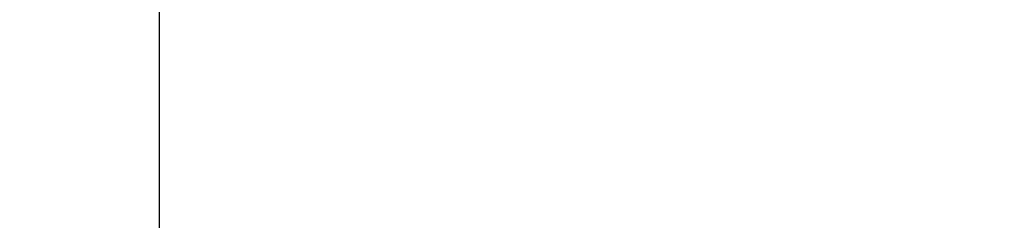
# Model space of a CAD drawing. Units: inches. Extents: x 2091 to 2899, y 967 to 2217.
# Tile 10 of 256: x 2312 to 2351, y 1080 to 1088. Entities that reach past the tile are written whole.
import ezdxf

# ---------------------------------------------------------------- set-up
doc = ezdxf.new("R2010")
doc.units = ezdxf.units.IN
doc.layers.add('A-ANNO-DIMS', color=2, linetype='Continuous', lineweight=18)
doc.styles.get("Standard").update_dxf_attribs({"font": 'arial.ttf'})
doc.dimstyles.new('ISO-25', dxfattribs={"dimtxt": 4, "dimasz": 4, "dimexe": 1.25, "dimexo": 0.625, "dimtad": 1, "dimdec": 0, "dimlunit": 3, "dimtxsty": 'Standard', "dimcen": 2.5, "dimadec": 0, "dimazin": 0, "dimtfac": 1, "dimtdec": 0, "dimtmove": 0, "dimatfit": 3, "dimfxl": 1, "dimarcsym": 0})

# ---------------------------------------------------------------- blocks, each defined once
blk = doc.blocks.new('*D68')
at = {"layer": 'A-ANNO-DIMS', "color": 0, "lineweight": -2, "transparency": 16777216}
for p, q in [((2317.144, 1535.794), (2317.144, 969.464)), ((2459.384, 1535.794), (2459.384, 969.464)), ((2321.144, 970.714), (2455.384, 970.714))]:
    blk.add_line(p, q, dxfattribs=at)
at = {"layer": 'A-ANNO-DIMS', "color": 0, "transparency": 16777216}
for points in [[(2321.144, 971.381), (2321.144, 970.048), (2317.144, 970.714)], [(2455.384, 971.381), (2455.384, 970.048), (2459.384, 970.714)]]:
    blk.add_solid(points, dxfattribs=at)
at = {"layer": 'Defpoints', "color": 0, "transparency": 16777216}
for p in [(2317.144, 1536.419), (2459.384, 1536.419), (2459.384, 970.714)]:
    blk.add_point(p, dxfattribs=at)
at = {"layer": 'A-ANNO-DIMS', "color": 0, "transparency": 16777216, "insert": (2388.264, 973.382), "char_height": 4, "attachment_point": 5}
blk.add_mtext('11\'-10"', dxfattribs=at)
blk = doc.blocks.new('*D71')
at = {"layer": 'A-ANNO-DIMS', "color": 0, "lineweight": -2, "transparency": 16777216}
for p, q in [((2212.144, 1351.294), (2212.144, 969.464)), ((2452.144, 1351.294), (2452.144, 969.464)), ((2216.144, 970.714), (2448.144, 970.714))]:
    blk.add_line(p, q, dxfattribs=at)
at = {"layer": 'A-ANNO-DIMS', "color": 0, "transparency": 16777216}
for points in [[(2216.144, 971.381), (2216.144, 970.048), (2212.144, 970.714)], [(2448.144, 971.381), (2448.144, 970.048), (2452.144, 970.714)]]:
    blk.add_solid(points, dxfattribs=at)
at = {"layer": 'Defpoints', "color": 0, "transparency": 16777216}
for p in [(2212.144, 1351.919), (2452.144, 1351.919), (2452.144, 970.714)]:
    blk.add_point(p, dxfattribs=at)
at = {"layer": 'A-ANNO-DIMS', "color": 0, "transparency": 16777216, "insert": (2332.144, 973.382), "char_height": 4, "attachment_point": 5}
blk.add_mtext('20\'-0"', dxfattribs=at)

msp = doc.modelspace()

# ---------------------------------------------------------------- dimensions: what is measured, and where the dimension line sits
at = {"layer": 'A-ANNO-DIMS'}
for base, p1, p2, picture, middle in [((2459.384, 970.714), (2317.144, 1536.419), (2459.384, 1536.419), '*D68', (2388.264, 973.382)), ((2452.144, 970.714), (2212.144, 1351.919), (2452.144, 1351.919), '*D71', (2332.144, 973.382))]:
    dim = msp.add_linear_dim(base=base, p1=p1, p2=p2, dimstyle='ISO-25', override={"dimdec": 1, "dimlfac": 1, "dimrnd": 0, "dimzin": 1, "dimdsep": 46, "dimlunit": 4, "dimfrac": 2}, dxfattribs=at)
    dim.commit()
    dim.dimension.update_dxf_attribs({"geometry": picture, "text_midpoint": middle})

doc.saveas('drawing.dxf')
